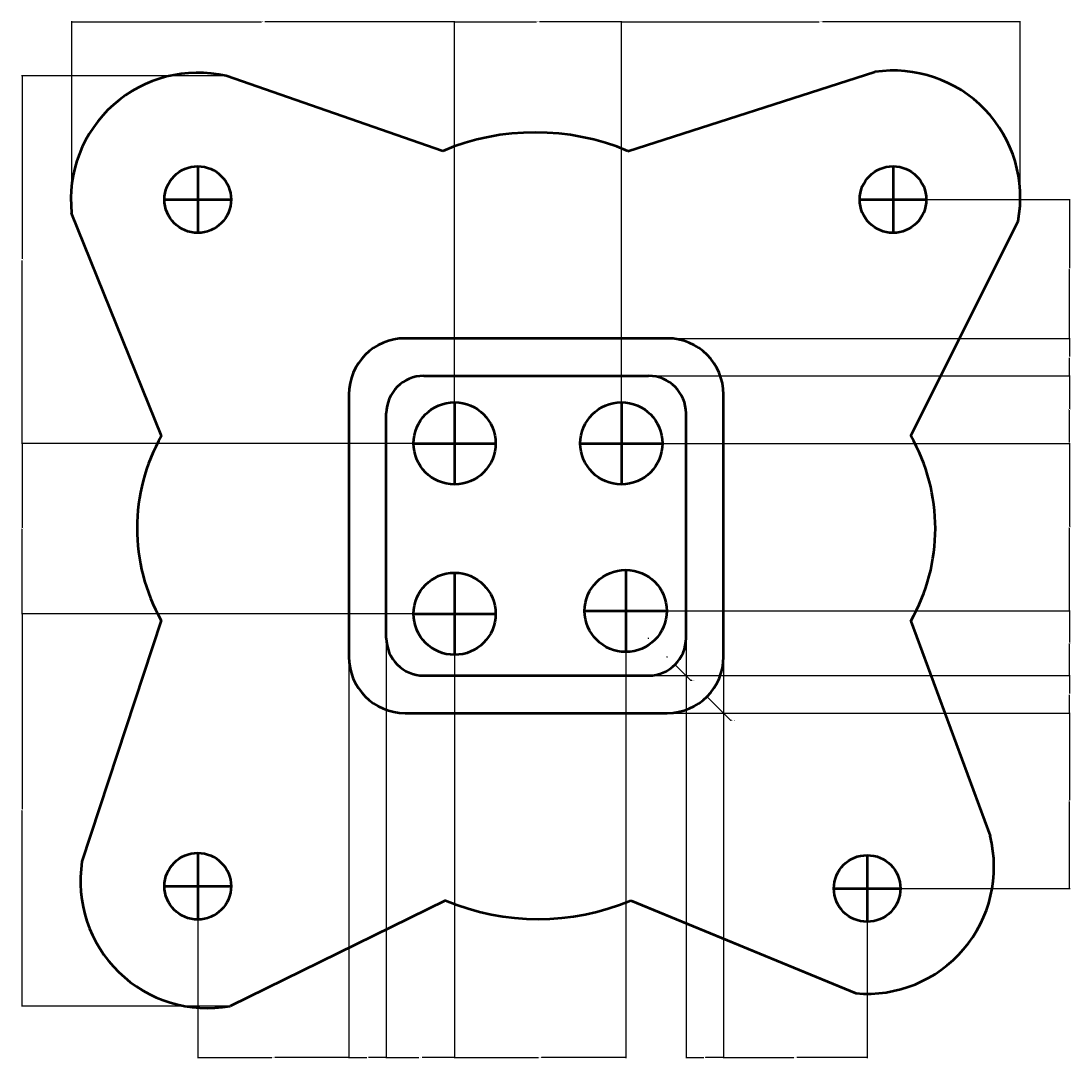
# Model space of a CAD drawing. Units: millimetres. Extents: x 2637 to 3282, y 1554 to 2264.
# Tile 1 of 3: x 2640 to 2920, y 1554 to 1831. Entities that reach past the tile are written whole.
import ezdxf

# ---------------------------------------------------------------- set-up
doc = ezdxf.new("R2010")
doc.units = ezdxf.units.MM
doc.layers.add('M-DIMS', color=2, linetype='Continuous', lineweight=18)
doc.layers.add('M-OUTL', color=7, linetype='Continuous', lineweight=50)
doc.styles.get("Standard").update_dxf_attribs({"font": 'arial.ttf'})
doc.dimstyles.get("Standard").update_dxf_attribs({"dimtxt": 0.18, "dimasz": 0.18, "dimexe": 0.18, "dimexo": 0.0625, "dimgap": 0.09, "dimtad": 0, "dimtih": 1, "dimtoh": 1, "dimdec": 4, "dimzin": 0, "dimdsep": 46, "dimtxsty": 'Standard', "dimcen": 0.09, "dimadec": 0, "dimazin": 0, "dimtfac": 1, "dimtdec": 4, "dimtofl": 0, "dimtmove": 0, "dimatfit": 3, "dimfxl": 1, "dimtolj": 1, "dimtzin": 0, "dimarcsym": 0})

# ---------------------------------------------------------------- blocks, each defined once
blk = doc.blocks.new('HOLE-MOUNT')
for p, q in [((2687.26, 1774.45), (2687.26, 1792.24)), ((2696.16, 1783.35), (2678.37, 1783.35))]:
    blk.add_line(p, q)
blk.add_circle((2687.26, 1783.35), 8.89)
blk = doc.blocks.new('HOLE-CENTRE')
for p, q in [((2755.81, 1707.32), (2755.81, 1729.25)), ((2766.78, 1718.29), (2744.85, 1718.29))]:
    blk.add_line(p, q)
blk.add_circle((2755.81, 1718.29), 10.96)
blk = doc.blocks.new('*D43')
at = {"layer": 'Defpoints', "color": 0, "transparency": 16777216}
for p in [(2755.81, 1830.83), (2653.7, 1787.8), (2755.81, 1718.29)]:
    blk.add_point(p, dxfattribs=at)
at = {"layer": 'M-DIMS', "color": 0, "lineweight": -2, "transparency": 16777216}
for p, q in [((2653.7, 1787.87), (2653.7, 1831.01)), ((2653.88, 1830.83), (2704.3, 1830.83)), ((2755.63, 1830.83), (2705.21, 1830.83)), ((2755.81, 1718.35), (2755.81, 1831.01))]:
    blk.add_line(p, q, dxfattribs=at)
at = {"layer": 'M-DIMS', "color": 0, "transparency": 16777216}
for points in [[(2653.88, 1830.86), (2653.88, 1830.8), (2653.7, 1830.83)], [(2755.63, 1830.86), (2755.63, 1830.8), (2755.81, 1830.83)]]:
    blk.add_solid(points, dxfattribs=at)
at = {"layer": 'M-DIMS', "color": 0, "transparency": 16777216, "insert": (2704.76, 1830.83), "char_height": 0.18, "attachment_point": 5}
blk.add_mtext('\\A1;102.12', dxfattribs=at)
blk = doc.blocks.new('*D44')
at = {"layer": 'Defpoints', "color": 0, "transparency": 16777216}
for p in [(2800.34, 1830.83), (2755.81, 1718.29), (2800.34, 1718.29)]:
    blk.add_point(p, dxfattribs=at)
at = {"layer": 'M-DIMS', "color": 0, "lineweight": -2, "transparency": 16777216}
for p, q in [((2755.81, 1718.35), (2755.81, 1831.01)), ((2755.99, 1830.83), (2777.68, 1830.83)), ((2800.16, 1830.83), (2778.47, 1830.83)), ((2800.34, 1718.35), (2800.34, 1831.01))]:
    blk.add_line(p, q, dxfattribs=at)
at = {"layer": 'M-DIMS', "color": 0, "transparency": 16777216}
for points in [[(2755.99, 1830.86), (2755.99, 1830.8), (2755.81, 1830.83)], [(2800.16, 1830.86), (2800.16, 1830.8), (2800.34, 1830.83)]]:
    blk.add_solid(points, dxfattribs=at)
at = {"layer": 'M-DIMS', "color": 0, "transparency": 16777216, "insert": (2778.08, 1830.83), "char_height": 0.18, "attachment_point": 5}
blk.add_mtext('\\A1;44.52', dxfattribs=at)
blk = doc.blocks.new('*D45')
at = {"layer": 'Defpoints', "color": 0, "transparency": 16777216}
for p in [(2906.77, 1830.83), (2906.77, 1785.7), (2800.34, 1718.29)]:
    blk.add_point(p, dxfattribs=at)
at = {"layer": 'M-DIMS', "color": 0, "lineweight": -2, "transparency": 16777216}
for p, q in [((2800.34, 1718.35), (2800.34, 1831.01)), ((2800.52, 1830.83), (2853.1, 1830.83)), ((2906.59, 1830.83), (2854.01, 1830.83)), ((2906.77, 1785.76), (2906.77, 1831.01))]:
    blk.add_line(p, q, dxfattribs=at)
at = {"layer": 'M-DIMS', "color": 0, "transparency": 16777216}
for points in [[(2800.52, 1830.86), (2800.52, 1830.8), (2800.34, 1830.83)], [(2906.59, 1830.86), (2906.59, 1830.8), (2906.77, 1830.83)]]:
    blk.add_solid(points, dxfattribs=at)
at = {"layer": 'M-DIMS', "color": 0, "transparency": 16777216, "insert": (2853.55, 1830.83), "char_height": 0.18, "attachment_point": 5}
blk.add_mtext('\\A1;106.43', dxfattribs=at)
blk = doc.blocks.new('*D46')
at = {"layer": 'Defpoints', "color": 0, "transparency": 16777216}
for p in [(2694.88, 1816.34), (2640.4, 1718.29), (2755.81, 1718.29)]:
    blk.add_point(p, dxfattribs=at)
at = {"layer": 'M-DIMS', "color": 0, "lineweight": -2, "transparency": 16777216}
for p, q in [((2694.82, 1816.34), (2640.22, 1816.34)), ((2640.4, 1816.16), (2640.4, 1767.5)), ((2640.4, 1718.47), (2640.4, 1767.13)), ((2755.75, 1718.29), (2640.22, 1718.29))]:
    blk.add_line(p, q, dxfattribs=at)
at = {"layer": 'M-DIMS', "color": 0, "transparency": 16777216}
for points in [[(2640.37, 1816.16), (2640.43, 1816.16), (2640.4, 1816.34)], [(2640.37, 1718.47), (2640.43, 1718.47), (2640.4, 1718.29)]]:
    blk.add_solid(points, dxfattribs=at)
at = {"layer": 'M-DIMS', "color": 0, "transparency": 16777216, "insert": (2640.4, 1767.32), "char_height": 0.18, "attachment_point": 5}
blk.add_mtext('\\A1;98.06', dxfattribs=at)
blk = doc.blocks.new('*D47')
at = {"layer": 'Defpoints', "color": 0, "transparency": 16777216}
for p in [(2755.81, 1718.29), (2640.4, 1672.8), (2755.81, 1672.8)]:
    blk.add_point(p, dxfattribs=at)
at = {"layer": 'M-DIMS', "color": 0, "lineweight": -2, "transparency": 16777216}
for p, q in [((2755.75, 1718.29), (2640.22, 1718.29)), ((2640.4, 1718.11), (2640.4, 1695.72)), ((2640.4, 1672.98), (2640.4, 1695.36)), ((2755.75, 1672.8), (2640.22, 1672.8))]:
    blk.add_line(p, q, dxfattribs=at)
at = {"layer": 'M-DIMS', "color": 0, "transparency": 16777216}
for points in [[(2640.37, 1718.11), (2640.43, 1718.11), (2640.4, 1718.29)], [(2640.37, 1672.98), (2640.43, 1672.98), (2640.4, 1672.8)]]:
    blk.add_solid(points, dxfattribs=at)
at = {"layer": 'M-DIMS', "color": 0, "transparency": 16777216, "insert": (2640.4, 1695.54), "char_height": 0.18, "attachment_point": 5}
blk.add_mtext('\\A1;45.49', dxfattribs=at)
blk = doc.blocks.new('*D48')
at = {"layer": 'Defpoints', "color": 0, "transparency": 16777216}
for p in [(2755.81, 1672.8), (2640.4, 1568.1), (2695.88, 1568.1)]:
    blk.add_point(p, dxfattribs=at)
at = {"layer": 'M-DIMS', "color": 0, "lineweight": -2, "transparency": 16777216}
for p, q in [((2755.75, 1672.8), (2640.22, 1672.8)), ((2640.4, 1672.62), (2640.4, 1620.63)), ((2640.4, 1568.28), (2640.4, 1620.27)), ((2695.81, 1568.1), (2640.22, 1568.1))]:
    blk.add_line(p, q, dxfattribs=at)
at = {"layer": 'M-DIMS', "color": 0, "transparency": 16777216}
for points in [[(2640.37, 1672.62), (2640.43, 1672.62), (2640.4, 1672.8)], [(2640.37, 1568.28), (2640.43, 1568.28), (2640.4, 1568.1)]]:
    blk.add_solid(points, dxfattribs=at)
at = {"layer": 'M-DIMS', "color": 0, "transparency": 16777216, "insert": (2640.4, 1620.45), "char_height": 0.18, "attachment_point": 5}
blk.add_mtext('\\A1;104.7', dxfattribs=at)
blk = doc.blocks.new('*D49')
at = {"layer": 'Defpoints', "color": 0, "transparency": 16777216}
for p in [(2727.6, 1661.31), (2687.26, 1600.08), (2727.6, 1554.41)]:
    blk.add_point(p, dxfattribs=at)
at = {"layer": 'M-DIMS', "color": 0, "lineweight": -2, "transparency": 16777216}
for p, q in [((2727.6, 1661.25), (2727.6, 1554.23)), ((2687.26, 1600.02), (2687.26, 1554.23)), ((2687.44, 1554.41), (2707.04, 1554.41)), ((2727.42, 1554.41), (2707.83, 1554.41))]:
    blk.add_line(p, q, dxfattribs=at)
at = {"layer": 'M-DIMS', "color": 0, "transparency": 16777216}
for points in [[(2687.44, 1554.44), (2687.44, 1554.38), (2687.26, 1554.41)], [(2727.42, 1554.44), (2727.42, 1554.38), (2727.6, 1554.41)]]:
    blk.add_solid(points, dxfattribs=at)
at = {"layer": 'M-DIMS', "color": 0, "transparency": 16777216, "insert": (2707.43, 1554.41), "char_height": 0.18, "attachment_point": 5}
blk.add_mtext('\\A1;40.34', dxfattribs=at)
blk = doc.blocks.new('*D50')
at = {"layer": 'Defpoints', "color": 0, "transparency": 16777216}
for p in [(2737.6, 1666.31), (2727.6, 1661.31), (2737.6, 1554.41)]:
    blk.add_point(p, dxfattribs=at)
at = {"layer": 'M-DIMS', "color": 0, "lineweight": -2, "transparency": 16777216}
for p, q in [((2737.6, 1666.25), (2737.6, 1554.23)), ((2727.6, 1661.25), (2727.6, 1554.23)), ((2727.78, 1554.41), (2732.39, 1554.41)), ((2737.42, 1554.41), (2732.81, 1554.41))]:
    blk.add_line(p, q, dxfattribs=at)
at = {"layer": 'M-DIMS', "color": 0, "transparency": 16777216}
for points in [[(2727.78, 1554.44), (2727.78, 1554.38), (2727.6, 1554.41)], [(2737.42, 1554.44), (2737.42, 1554.38), (2737.6, 1554.41)]]:
    blk.add_solid(points, dxfattribs=at)
at = {"layer": 'M-DIMS', "color": 0, "transparency": 16777216, "insert": (2732.6, 1554.41), "char_height": 0.18, "attachment_point": 5}
blk.add_mtext('\\A1;10', dxfattribs=at)
blk = doc.blocks.new('*D51')
at = {"layer": 'Defpoints', "color": 0, "transparency": 16777216}
for p in [(2755.81, 1672.8), (2737.6, 1666.31), (2755.81, 1554.41)]:
    blk.add_point(p, dxfattribs=at)
at = {"layer": 'M-DIMS', "color": 0, "lineweight": -2, "transparency": 16777216}
for p, q in [((2755.81, 1672.74), (2755.81, 1554.23)), ((2737.6, 1666.25), (2737.6, 1554.23)), ((2737.78, 1554.41), (2746.25, 1554.41)), ((2755.63, 1554.41), (2747.16, 1554.41))]:
    blk.add_line(p, q, dxfattribs=at)
at = {"layer": 'M-DIMS', "color": 0, "transparency": 16777216}
for points in [[(2737.78, 1554.44), (2737.78, 1554.38), (2737.6, 1554.41)], [(2755.63, 1554.44), (2755.63, 1554.38), (2755.81, 1554.41)]]:
    blk.add_solid(points, dxfattribs=at)
at = {"layer": 'M-DIMS', "color": 0, "transparency": 16777216, "insert": (2746.71, 1554.41), "char_height": 0.18, "attachment_point": 5}
blk.add_mtext('\\A1;18.212', dxfattribs=at)
blk = doc.blocks.new('*D52')
at = {"layer": 'Defpoints', "color": 0, "transparency": 16777216}
for p in [(2801.49, 1673.57), (2755.81, 1672.8), (2801.49, 1554.41)]:
    blk.add_point(p, dxfattribs=at)
at = {"layer": 'M-DIMS', "color": 0, "lineweight": -2, "transparency": 16777216}
for p, q in [((2801.49, 1673.51), (2801.49, 1554.23)), ((2755.81, 1672.74), (2755.81, 1554.23)), ((2755.99, 1554.41), (2778.26, 1554.41)), ((2801.31, 1554.41), (2779.05, 1554.41))]:
    blk.add_line(p, q, dxfattribs=at)
at = {"layer": 'M-DIMS', "color": 0, "transparency": 16777216}
for points in [[(2755.99, 1554.44), (2755.99, 1554.38), (2755.81, 1554.41)], [(2801.31, 1554.44), (2801.31, 1554.38), (2801.49, 1554.41)]]:
    blk.add_solid(points, dxfattribs=at)
at = {"layer": 'M-DIMS', "color": 0, "transparency": 16777216, "insert": (2778.65, 1554.41), "char_height": 0.18, "attachment_point": 5}
blk.add_mtext('\\A1;45.68', dxfattribs=at)
blk = doc.blocks.new('*D53')
at = {"layer": 'Defpoints', "color": 0, "transparency": 16777216}
for p in [(2817.6, 1666.31), (2827.6, 1661.31), (2827.6, 1554.41)]:
    blk.add_point(p, dxfattribs=at)
at = {"layer": 'M-DIMS', "color": 0, "lineweight": -2, "transparency": 16777216}
for p, q in [((2817.6, 1666.25), (2817.6, 1554.23)), ((2827.6, 1661.25), (2827.6, 1554.23)), ((2817.78, 1554.41), (2822.39, 1554.41)), ((2827.42, 1554.41), (2822.81, 1554.41))]:
    blk.add_line(p, q, dxfattribs=at)
at = {"layer": 'M-DIMS', "color": 0, "transparency": 16777216}
for points in [[(2817.78, 1554.44), (2817.78, 1554.38), (2817.6, 1554.41)], [(2827.42, 1554.44), (2827.42, 1554.38), (2827.6, 1554.41)]]:
    blk.add_solid(points, dxfattribs=at)
at = {"layer": 'M-DIMS', "color": 0, "transparency": 16777216, "insert": (2822.6, 1554.41), "char_height": 0.18, "attachment_point": 5}
blk.add_mtext('\\A1;10', dxfattribs=at)
blk = doc.blocks.new('*D54')
at = {"layer": 'Defpoints', "color": 0, "transparency": 16777216}
for p in [(2827.6, 1661.31), (2865.94, 1599.48), (2865.94, 1554.41)]:
    blk.add_point(p, dxfattribs=at)
at = {"layer": 'M-DIMS', "color": 0, "lineweight": -2, "transparency": 16777216}
for p, q in [((2827.6, 1661.25), (2827.6, 1554.23)), ((2865.94, 1599.42), (2865.94, 1554.23)), ((2827.78, 1554.41), (2846.38, 1554.41)), ((2865.76, 1554.41), (2847.16, 1554.41))]:
    blk.add_line(p, q, dxfattribs=at)
at = {"layer": 'M-DIMS', "color": 0, "transparency": 16777216}
for points in [[(2827.78, 1554.44), (2827.78, 1554.38), (2827.6, 1554.41)], [(2865.76, 1554.44), (2865.76, 1554.38), (2865.94, 1554.41)]]:
    blk.add_solid(points, dxfattribs=at)
at = {"layer": 'M-DIMS', "color": 0, "transparency": 16777216, "insert": (2846.77, 1554.41), "char_height": 0.18, "attachment_point": 5}
blk.add_mtext('\\A1;38.34', dxfattribs=at)
blk = doc.blocks.new('*D55')
at = {"layer": 'Defpoints', "color": 0, "transparency": 16777216}
for p in [(2872.83, 1783.35), (2812.6, 1746.31), (2919.97, 1746.31)]:
    blk.add_point(p, dxfattribs=at)
at = {"layer": 'M-DIMS', "color": 0, "lineweight": -2, "transparency": 16777216}
for p, q in [((2872.9, 1783.35), (2920.15, 1783.35)), ((2919.97, 1783.17), (2919.97, 1765.01)), ((2919.97, 1746.49), (2919.97, 1764.65)), ((2812.66, 1746.31), (2920.15, 1746.31))]:
    blk.add_line(p, q, dxfattribs=at)
at = {"layer": 'M-DIMS', "color": 0, "transparency": 16777216}
for points in [[(2919.94, 1783.17), (2920, 1783.17), (2919.97, 1783.35)], [(2919.94, 1746.49), (2920, 1746.49), (2919.97, 1746.31)]]:
    blk.add_solid(points, dxfattribs=at)
at = {"layer": 'M-DIMS', "color": 0, "transparency": 16777216, "insert": (2919.97, 1764.83), "char_height": 0.18, "attachment_point": 5}
blk.add_mtext('\\A1;37.04', dxfattribs=at)
blk = doc.blocks.new('*D56')
at = {"layer": 'Defpoints', "color": 0, "transparency": 16777216}
for p in [(2812.6, 1746.31), (2807.6, 1736.31), (2919.97, 1736.31)]:
    blk.add_point(p, dxfattribs=at)
at = {"layer": 'M-DIMS', "color": 0, "lineweight": -2, "transparency": 16777216}
for p, q in [((2812.66, 1746.31), (2920.15, 1746.31)), ((2919.97, 1746.13), (2919.97, 1741.49)), ((2919.97, 1736.49), (2919.97, 1741.13)), ((2807.66, 1736.31), (2920.15, 1736.31))]:
    blk.add_line(p, q, dxfattribs=at)
at = {"layer": 'M-DIMS', "color": 0, "transparency": 16777216}
for points in [[(2919.94, 1746.13), (2920, 1746.13), (2919.97, 1746.31)], [(2919.94, 1736.49), (2920, 1736.49), (2919.97, 1736.31)]]:
    blk.add_solid(points, dxfattribs=at)
at = {"layer": 'M-DIMS', "color": 0, "transparency": 16777216, "insert": (2919.97, 1741.31), "char_height": 0.18, "attachment_point": 5}
blk.add_mtext('\\A1;10', dxfattribs=at)
blk = doc.blocks.new('*D57')
at = {"layer": 'Defpoints', "color": 0, "transparency": 16777216}
for p in [(2807.6, 1736.31), (2800.34, 1718.29), (2919.97, 1718.29)]:
    blk.add_point(p, dxfattribs=at)
at = {"layer": 'M-DIMS', "color": 0, "lineweight": -2, "transparency": 16777216}
for p, q in [((2807.66, 1736.31), (2920.15, 1736.31)), ((2919.97, 1736.13), (2919.97, 1727.48)), ((2919.97, 1718.47), (2919.97, 1727.12)), ((2800.4, 1718.29), (2920.15, 1718.29))]:
    blk.add_line(p, q, dxfattribs=at)
at = {"layer": 'M-DIMS', "color": 0, "transparency": 16777216}
for points in [[(2919.94, 1736.13), (2920, 1736.13), (2919.97, 1736.31)], [(2919.94, 1718.47), (2920, 1718.47), (2919.97, 1718.29)]]:
    blk.add_solid(points, dxfattribs=at)
at = {"layer": 'M-DIMS', "color": 0, "transparency": 16777216, "insert": (2919.97, 1727.3), "char_height": 0.18, "attachment_point": 5}
blk.add_mtext('\\A1;18.024', dxfattribs=at)
blk = doc.blocks.new('*D58')
at = {"layer": 'Defpoints', "color": 0, "transparency": 16777216}
for p in [(2800.34, 1718.29), (2801.49, 1673.57), (2919.97, 1673.57)]:
    blk.add_point(p, dxfattribs=at)
at = {"layer": 'M-DIMS', "color": 0, "lineweight": -2, "transparency": 16777216}
for p, q in [((2800.4, 1718.29), (2920.15, 1718.29)), ((2919.97, 1718.11), (2919.97, 1696.11)), ((2919.97, 1673.75), (2919.97, 1695.75)), ((2801.56, 1673.57), (2920.15, 1673.57))]:
    blk.add_line(p, q, dxfattribs=at)
at = {"layer": 'M-DIMS', "color": 0, "transparency": 16777216}
for points in [[(2919.94, 1718.11), (2920, 1718.11), (2919.97, 1718.29)], [(2919.94, 1673.75), (2920, 1673.75), (2919.97, 1673.57)]]:
    blk.add_solid(points, dxfattribs=at)
at = {"layer": 'M-DIMS', "color": 0, "transparency": 16777216, "insert": (2919.97, 1695.93), "char_height": 0.18, "attachment_point": 5}
blk.add_mtext('\\A1;44.72', dxfattribs=at)
blk = doc.blocks.new('*D59')
at = {"layer": 'Defpoints', "color": 0, "transparency": 16777216}
for p in [(2801.49, 1673.57), (2807.6, 1656.31), (2919.97, 1656.31)]:
    blk.add_point(p, dxfattribs=at)
at = {"layer": 'M-DIMS', "color": 0, "lineweight": -2, "transparency": 16777216}
for p, q in [((2801.56, 1673.57), (2920.15, 1673.57)), ((2919.97, 1673.39), (2919.97, 1665.12)), ((2919.97, 1656.49), (2919.97, 1664.76)), ((2807.66, 1656.31), (2920.15, 1656.31))]:
    blk.add_line(p, q, dxfattribs=at)
at = {"layer": 'M-DIMS', "color": 0, "transparency": 16777216}
for points in [[(2919.94, 1673.39), (2920, 1673.39), (2919.97, 1673.57)], [(2919.94, 1656.49), (2920, 1656.49), (2919.97, 1656.31)]]:
    blk.add_solid(points, dxfattribs=at)
at = {"layer": 'M-DIMS', "color": 0, "transparency": 16777216, "insert": (2919.97, 1664.94), "char_height": 0.18, "attachment_point": 5}
blk.add_mtext('\\A1;17.26', dxfattribs=at)
blk = doc.blocks.new('*D60')
at = {"layer": 'Defpoints', "color": 0, "transparency": 16777216}
for p in [(2807.6, 1656.31), (2812.6, 1646.31), (2919.97, 1646.31)]:
    blk.add_point(p, dxfattribs=at)
at = {"layer": 'M-DIMS', "color": 0, "lineweight": -2, "transparency": 16777216}
for p, q in [((2807.66, 1656.31), (2920.15, 1656.31)), ((2919.97, 1656.13), (2919.97, 1651.49)), ((2919.97, 1646.49), (2919.97, 1651.13)), ((2812.66, 1646.31), (2920.15, 1646.31))]:
    blk.add_line(p, q, dxfattribs=at)
at = {"layer": 'M-DIMS', "color": 0, "transparency": 16777216}
for points in [[(2919.94, 1656.13), (2920, 1656.13), (2919.97, 1656.31)], [(2919.94, 1646.49), (2920, 1646.49), (2919.97, 1646.31)]]:
    blk.add_solid(points, dxfattribs=at)
at = {"layer": 'M-DIMS', "color": 0, "transparency": 16777216, "insert": (2919.97, 1651.31), "char_height": 0.18, "attachment_point": 5}
blk.add_mtext('\\A1;10', dxfattribs=at)
blk = doc.blocks.new('*D61')
at = {"layer": 'Defpoints', "color": 0, "transparency": 16777216}
for p in [(2812.6, 1646.31), (2865.94, 1599.48), (2919.97, 1599.48)]:
    blk.add_point(p, dxfattribs=at)
at = {"layer": 'M-DIMS', "color": 0, "lineweight": -2, "transparency": 16777216}
for p, q in [((2812.66, 1646.31), (2920.15, 1646.31)), ((2919.97, 1646.13), (2919.97, 1623.08)), ((2919.97, 1599.66), (2919.97, 1622.71)), ((2866, 1599.48), (2920.15, 1599.48))]:
    blk.add_line(p, q, dxfattribs=at)
at = {"layer": 'M-DIMS', "color": 0, "transparency": 16777216}
for points in [[(2919.94, 1646.13), (2920, 1646.13), (2919.97, 1646.31)], [(2919.94, 1599.66), (2920, 1599.66), (2919.97, 1599.48)]]:
    blk.add_solid(points, dxfattribs=at)
at = {"layer": 'M-DIMS', "color": 0, "transparency": 16777216, "insert": (2919.97, 1622.9), "char_height": 0.18, "attachment_point": 5}
blk.add_mtext('\\A1;46.83', dxfattribs=at)
blk = doc.blocks.new('*D69')
at = {"layer": 'Defpoints', "color": 0, "transparency": 16777216}
for p in [(2812.6, 1661.31), (2823.21, 1650.7)]:
    blk.add_point(p, dxfattribs=at)
at = {"layer": 'M-DIMS', "color": 0, "lineweight": -2, "transparency": 16777216}
for p, q in [((2812.51, 1661.31), (2812.69, 1661.31)), ((2812.6, 1661.22), (2812.6, 1661.4)), ((2829.57, 1644.34), (2823.34, 1650.58)), ((2829.75, 1644.34), (2829.57, 1644.34))]:
    blk.add_line(p, q, dxfattribs=at)
at = {"layer": 'M-DIMS', "color": 0, "transparency": 16777216}
blk.add_solid([(2823.36, 1650.6), (2823.31, 1650.56), (2823.21, 1650.7)], dxfattribs=at)
at = {"layer": 'M-DIMS', "color": 0, "transparency": 16777216, "insert": (2830.26, 1644.34), "char_height": 0.18, "attachment_point": 5}
blk.add_mtext('\\A1;4X R15', dxfattribs=at)
blk = doc.blocks.new('*D70')
at = {"layer": 'Defpoints', "color": 0, "transparency": 16777216}
for p in [(2807.6, 1666.31), (2814.67, 1659.24)]:
    blk.add_point(p, dxfattribs=at)
at = {"layer": 'M-DIMS', "color": 0, "lineweight": -2, "transparency": 16777216}
for p, q in [((2807.51, 1666.31), (2807.69, 1666.31)), ((2807.6, 1666.22), (2807.6, 1666.4)), ((2818.92, 1655), (2814.8, 1659.11)), ((2819.1, 1655), (2818.92, 1655))]:
    blk.add_line(p, q, dxfattribs=at)
at = {"layer": 'M-DIMS', "color": 0, "transparency": 16777216}
blk.add_solid([(2814.82, 1659.13), (2814.78, 1659.09), (2814.67, 1659.24)], dxfattribs=at)
at = {"layer": 'M-DIMS', "color": 0, "transparency": 16777216, "insert": (2819.6, 1655), "char_height": 0.18, "attachment_point": 5}
blk.add_mtext('\\A1;4X R10', dxfattribs=at)

msp = doc.modelspace()

# ---------------------------------------------------------------- linework, layer by layer
at = {"layer": 'M-OUTL'}
for p, q in [((2752.6515, 1796.3103), (2694.8776, 1816.3435)), ((2802.0818, 1796.3103), (2867.9757, 1817.4088)), ((2677.6018, 1720.2903), (2653.599, 1779.7019)), ((2877.6018, 1720.2903), (2906.2275, 1777.6178)), ((2812.6018, 1746.3103), (2742.6018, 1746.3103)), ((2747.6018, 1736.3103), (2807.6018, 1736.3103)), ((2817.6018, 1736.3103), (2817.6018, 1736.3103)), ((2727.6018, 1731.3103), (2727.6018, 1661.3103)), ((2827.6018, 1661.3103), (2827.6018, 1731.3103)), ((2737.6018, 1666.3103), (2737.6018, 1726.3103)), ((2817.6018, 1666.3103), (2817.6018, 1726.3103)), ((2677.4992, 1671.0414), (2656.3637, 1606.6377)), ((2877.6018, 1670.8603), (2898.7651, 1613.4907)), ((2747.6018, 1656.3103), (2807.6018, 1656.3103)), ((2742.6018, 1646.3103), (2812.6018, 1646.3103)), ((2753.4101, 1596.3103), (2695.8773, 1568.0994)), ((2802.8405, 1596.3103), (2862.9407, 1571.501))]:
    msp.add_line(p, q, dxfattribs=at)
for centre, radius, start, end in [((2687.264, 1783.3486), 33.8619, 77.006317, 186.182441), ((2872.9563, 1783.9152), 33.8619, 349.282109, 98.458233), ((2777.3666, 1737.4311), 63.856, 67.229222, 112.770778), ((2777.3666, 1737.4311), 63.856, 67.229222, 112.770778), ((2742.6018, 1731.3103), 15, 90, 180), ((2812.6018, 1731.3103), 15, 0, 90), ((2747.6018, 1726.3103), 10, 90, 180), ((2807.6018, 1726.3103), 10, 0, 90), ((2721.0132, 1695.5753), 49.9538, 150.346232, 209.414951), ((2834.1905, 1695.5753), 49.9538, 330.346232, 29.653768), ((2747.6018, 1666.3103), 10, 180, 270), ((2807.6018, 1666.3103), 10, 270, 0), ((2742.6018, 1661.3103), 15, 180, 270), ((2812.6018, 1661.3103), 15, 270, 0), ((2865.926, 1605.231), 33.8619, 264.94216, 14.118284), ((2689.8204, 1601.4152), 33.8619, 171.127908, 280.304032), ((2778.1253, 1655.1894), 63.856, 247.229222, 292.770778)]:
    msp.add_arc(centre, radius, start, end, dxfattribs=at)

# ---------------------------------------------------------------- block references
at = {"layer": 'M-OUTL', "rotation": 180}
for name, p in [('HOLE-MOUNT', (5374.5279, 3566.6973)), ('HOLE-MOUNT', (5560.0987, 3566.6973)), ('HOLE-CENTRE', (5511.6285, 3436.5732)), ('HOLE-CENTRE', (5556.1514, 3436.5732)), ('HOLE-CENTRE', (5557.3092, 3391.8566)), ('HOLE-CENTRE', (5511.6285, 3391.0858)), ('HOLE-MOUNT', (5374.5279, 3383.4288)), ('HOLE-MOUNT', (5553.2044, 3382.8311))]:
    msp.add_blockref(name, p, dxfattribs=at)

# ---------------------------------------------------------------- dimensions: what is measured, and where the dimension line sits
at = {"layer": 'M-DIMS'}
for base, p1, p2, override, picture, middle in [((2755.8142, 1830.8337), (2653.6959, 1787.8029), (2755.8142, 1718.2866), {"dimdec": 2, "dimlfac": 1, "dimrnd": 0, "dimzin": 0, "dimdsep": 46, "dimlunit": 2}, '*D43', (2704.7551, 1830.8337)), ((2800.3371, 1830.8337), (2755.8142, 1718.2866), (2800.3371, 1718.2866), {"dimdec": 2, "dimlfac": 1, "dimrnd": 0, "dimzin": 0, "dimdsep": 46, "dimlunit": 2}, '*D44', (2778.0757, 1830.8337)), ((2906.7715, 1830.8337), (2800.3371, 1718.2866), (2906.7715, 1785.7011), {"dimdec": 2, "dimlfac": 1, "dimrnd": 0, "dimzin": 0, "dimdsep": 46, "dimlunit": 2}, '*D45', (2853.5543, 1830.8337)), ((2801.4949, 1554.4138), (2755.8142, 1672.7992), (2801.4949, 1673.57), {"dimdec": 2, "dimlfac": 1, "dimrnd": 0, "dimzin": 0, "dimdsep": 46, "dimlunit": 2}, '*D52', (2778.6546, 1554.4138)), ((2755.8142, 1554.4138), (2737.6018, 1666.3103), (2755.8142, 1672.7992), {"dimdec": 3, "dimlfac": 1, "dimrnd": 0, "dimzin": 0, "dimdsep": 46, "dimlunit": 2}, '*D51', (2746.708, 1554.4138)), ((2737.6018, 1554.4138), (2727.6018, 1661.3103), (2737.6018, 1666.3103), {"dimdec": 0, "dimlfac": 1, "dimrnd": 0, "dimzin": 0, "dimdsep": 46, "dimlunit": 2}, '*D50', (2732.6018, 1554.4138)), ((2827.6018, 1554.4138), (2817.6018, 1666.3103), (2827.6018, 1661.3103), {"dimdec": 0, "dimlfac": 1, "dimrnd": 0, "dimzin": 0, "dimdsep": 46, "dimlunit": 2}, '*D53', (2822.6018, 1554.4138)), ((2727.6018, 1554.4138), (2687.264, 1600.0801), (2727.6018, 1661.3103), {"dimdec": 2, "dimlfac": 1, "dimrnd": 0, "dimzin": 0, "dimdsep": 46, "dimlunit": 2}, '*D49', (2707.4329, 1554.4138)), ((2865.9404, 1554.4138), (2827.6018, 1661.3103), (2865.9404, 1599.4825), {"dimdec": 2, "dimlfac": 1, "dimrnd": 0, "dimzin": 0, "dimdsep": 46, "dimlunit": 2}, '*D54', (2846.7711, 1554.4138))]:
    dim = msp.add_linear_dim(base=base, p1=p1, p2=p2, dimstyle='Standard', override=override, dxfattribs=at)
    dim.commit()
    dim.dimension.update_dxf_attribs({"geometry": picture, "text_midpoint": middle})
for base, p1, p2, override, picture, middle in [((2640.399, 1718.2866), (2694.8776, 1816.3435), (2755.8142, 1718.2866), {"dimdec": 2, "dimlfac": 1, "dimrnd": 0, "dimzin": 0, "dimdsep": 46, "dimlunit": 2}, '*D46', (2640.399, 1767.315)), ((2919.9715, 1746.3103), (2872.8348, 1783.3486), (2812.6018, 1746.3103), {"dimdec": 2, "dimlfac": 1, "dimrnd": 0, "dimzin": 0, "dimdsep": 46, "dimlunit": 2}, '*D55', (2919.9715, 1764.8295)), ((2919.9715, 1736.3103), (2812.6018, 1746.3103), (2807.6018, 1736.3103), {"dimdec": 0, "dimlfac": 1, "dimrnd": 0, "dimzin": 0, "dimdsep": 46, "dimlunit": 2}, '*D56', (2919.9715, 1741.3103)), ((2919.9715, 1718.2866), (2807.6018, 1736.3103), (2800.3371, 1718.2866), {"dimdec": 3, "dimlfac": 1, "dimrnd": 0, "dimzin": 0, "dimdsep": 46, "dimlunit": 2}, '*D57', (2919.9715, 1727.2984)), ((2640.399, 1672.7992), (2755.8142, 1718.2866), (2755.8142, 1672.7992), {"dimdec": 2, "dimlfac": 1, "dimrnd": 0, "dimzin": 0, "dimdsep": 46, "dimlunit": 2}, '*D47', (2640.399, 1695.5429)), ((2919.9715, 1673.57), (2800.3371, 1718.2866), (2801.4949, 1673.57), {"dimdec": 2, "dimlfac": 1, "dimrnd": 0, "dimzin": 0, "dimdsep": 46, "dimlunit": 2}, '*D58', (2919.9715, 1695.9283)), ((2919.9715, 1656.3103), (2801.4949, 1673.57), (2807.6018, 1656.3103), {"dimdec": 2, "dimlfac": 1, "dimrnd": 0, "dimzin": 0, "dimdsep": 46, "dimlunit": 2}, '*D59', (2919.9715, 1664.9401)), ((2640.399, 1568.0994), (2755.8142, 1672.7992), (2695.8773, 1568.0994), {"dimdec": 1, "dimlfac": 1, "dimrnd": 0, "dimzin": 0, "dimdsep": 46, "dimlunit": 2}, '*D48', (2640.399, 1620.4493)), ((2919.9715, 1646.3103), (2807.6018, 1656.3103), (2812.6018, 1646.3103), {"dimdec": 0, "dimlfac": 1, "dimrnd": 0, "dimzin": 0, "dimdsep": 46, "dimlunit": 2}, '*D60', (2919.9715, 1651.3103)), ((2919.9715, 1599.4825), (2812.6018, 1646.3103), (2865.9404, 1599.4825), {"dimdec": 2, "dimlfac": 1, "dimrnd": 0, "dimzin": 0, "dimdsep": 46, "dimlunit": 2}, '*D61', (2919.9715, 1622.8964))]:
    dim = msp.add_linear_dim(base=base, p1=p1, p2=p2, angle=90, dimstyle='Standard', override=override, dxfattribs=at)
    dim.commit()
    dim.dimension.update_dxf_attribs({"geometry": picture, "text_midpoint": middle})
for center, mpoint, picture, middle in [((2807.6018, 1666.3103), (2814.6728, 1659.2392), '*D70', (2819.5972, 1654.9965)), ((2812.6018, 1661.3103), (2823.2084, 1650.7036), '*D69', (2830.255, 1644.3396))]:
    dim = msp.add_radius_dim(center=center, mpoint=mpoint, text='4X <>', dimstyle='Standard', override={"dimdec": 0, "dimlfac": 1, "dimrnd": 0, "dimzin": 0, "dimdsep": 46, "dimlunit": 2}, dxfattribs=at)
    dim.commit()
    dim.dimension.update_dxf_attribs({"geometry": picture, "text_midpoint": middle, "dimtype": 164})

doc.saveas('drawing.dxf')
